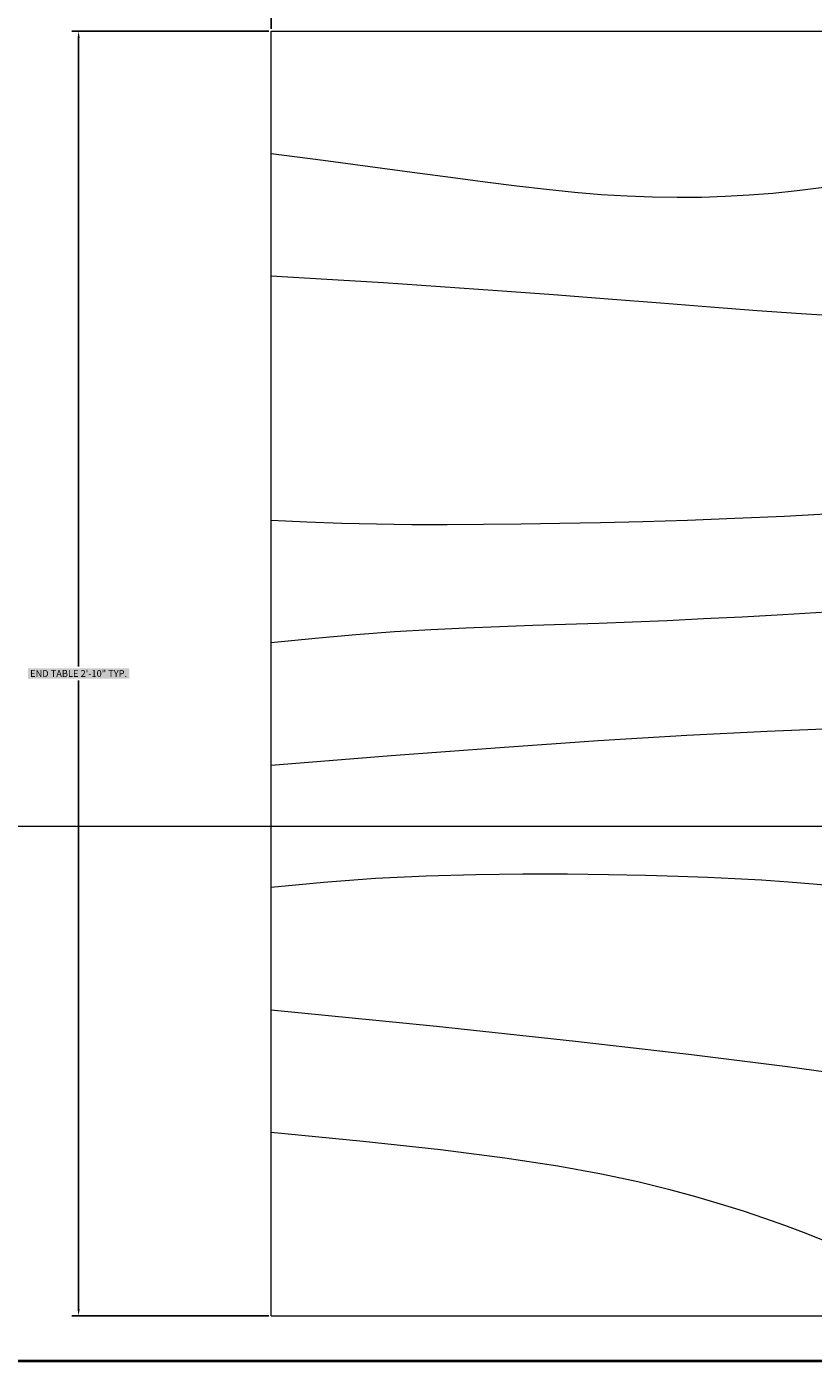
# Model space of a CAD drawing. Units: inches. Extents: x -301 to 715, y -607 to 364.
# Tile 100 of 141: x 82 to 103, y -10 to 26. Entities that reach past the tile are written whole.
import ezdxf

# ---------------------------------------------------------------- set-up
doc = ezdxf.new("R2010")
doc.units = ezdxf.units.IN
doc.header["$MEASUREMENT"] = 0
for name, color, linetype, lineweight in [('A-ANNO-DIMS', 2, 'Continuous', 18), ('A-FURN', 8, 'Continuous', 18), ('A-WALL', 3, 'Continuous', 40)]:
    doc.layers.add(name, color=color, linetype=linetype, lineweight=lineweight)
doc.styles.get("Standard").update_dxf_attribs({"font": 'arial.ttf'})
doc.dimstyles.get("Standard").update_dxf_attribs({"dimtxt": 0.18, "dimasz": 0.18, "dimexe": 0.18, "dimexo": 0.0625, "dimgap": 0.09, "dimtad": 0, "dimtih": 1, "dimtoh": 1, "dimdec": 1, "dimzin": 0, "dimdsep": 46, "dimlunit": 4, "dimtxsty": 'Standard', "dimcen": 0.09, "dimclrd": 3, "dimclre": 4, "dimclrt": 6, "dimadec": 0, "dimazin": 0, "dimtfac": 1, "dimtdec": 1, "dimtofl": 0, "dimtmove": 0, "dimatfit": 3, "dimfxl": 1, "dimtfill": 2, "dimtfillclr": 51, "dimtolj": 1, "dimtzin": 0, "dimarcsym": 0})

# ---------------------------------------------------------------- blocks, each defined once
blk = doc.blocks.new('Table - Square Woodgrain 42 x 42 in.')
blk.add_line((0, -42), (42, -42))
for points in [[(0, -4), (1.704, -4.2172), (3.2358, -4.4188), (4.615, -4.604), (5.8615, -4.7721), (6.9951, -4.9224), (8.0357, -5.0541), (9.0031, -5.1667), (9.9171, -5.2594), (10.7951, -5.3316), (11.6445, -5.3836), (12.4702, -5.4157), (13.277, -5.4283), (14.0698, -5.4217), (14.8535, -5.3964), (15.6331, -5.3526), (16.4133, -5.2908), (17.1986, -5.2103), (17.9913, -5.1062), (18.793, -4.9727), (19.6056, -4.8038), (20.4307, -4.5937), (21.2701, -4.3365), (22.1256, -4.0262), (22.9989, -3.6571), (23.888, -3.2272), (24.7756, -2.7516), (25.6408, -2.2491), (26.4624, -1.7387), (27.2195, -1.2395), (27.891, -0.7703), (28.456, -0.3501), (28.8934, 0.002)], [(0, -42), (0, 0), (42, 0), (42, -42)], [(0, -8), (1.8203, -8.1001), (3.6741, -8.2149), (5.5411, -8.3408), (7.4011, -8.4741), (9.2339, -8.6112), (11.0193, -8.7484), (12.7371, -8.8821), (14.3671, -9.0086), (15.8954, -9.1246), (17.3337, -9.2278), (18.6997, -9.3159), (20.0116, -9.387), (21.2871, -9.4389), (22.5442, -9.4696), (23.8008, -9.477), (25.0749, -9.459), (26.3791, -9.4137), (27.7049, -9.3403), (29.0383, -9.2382), (30.3655, -9.1068), (31.6728, -8.9455), (32.9461, -8.7535), (34.1717, -8.5304), (35.3358, -8.2756), (36.4268, -7.9863), (37.443, -7.6521), (38.3849, -7.2603), (39.253, -6.7986), (40.048, -6.2542), (40.7705, -5.6147), (41.421, -4.8674), (42, -4)], [(42, -12), (39.1784, -12.8621), (36.4519, -13.5654), (33.8246, -14.1294), (31.3004, -14.5731), (28.8832, -14.9161), (26.577, -15.1775), (24.3858, -15.3768), (22.3136, -15.5332), (20.3622, -15.6632), (18.5254, -15.7718), (16.7947, -15.8612), (15.1618, -15.9338), (13.6183, -15.9916), (12.1558, -16.0369), (10.7659, -16.0718), (9.4403, -16.0987), (8.1703, -16.1191), (6.9461, -16.1325), (5.7577, -16.1377), (4.595, -16.1335), (3.4479, -16.1188), (2.3064, -16.0924), (1.1604, -16.0532), (0, -16)], [(42, -16), (37.6529, -16.7365), (33.8802, -17.329), (30.6179, -17.7961), (27.8015, -18.1561), (25.3668, -18.4275), (23.2497, -18.6288), (21.3859, -18.7785), (19.7111, -18.8949), (18.1693, -18.9939), (16.7375, -19.0795), (15.401, -19.1534), (14.1449, -19.217), (12.9544, -19.2717), (11.8148, -19.3191), (10.7113, -19.3606), (9.6291, -19.3976), (8.5534, -19.4323), (7.47, -19.4689), (6.3643, -19.5122), (5.222, -19.5672), (4.0288, -19.6386), (2.7703, -19.7313), (1.4321, -19.8501), (0, -20)], [(0, -24), (3.9243, -23.6805), (7.4766, -23.4138), (10.6891, -23.1954), (13.5943, -23.0205), (16.2247, -22.8847), (18.6125, -22.7832), (20.7903, -22.7116), (22.7903, -22.6651), (24.6563, -22.642), (26.4764, -22.6507), (28.35, -22.7024), (30.3766, -22.8084), (32.6555, -22.98), (35.2861, -23.2283), (38.3678, -23.5645), (42, -24)], [(42, -32), (37.392, -31.017), (33.4585, -30.2231), (30.1291, -29.5949), (27.3334, -29.109), (25.0009, -28.742), (23.0612, -28.4707), (21.4439, -28.2716), (20.0786, -28.1215), (18.8998, -28.0002), (17.8609, -27.9014), (16.9206, -27.8219), (16.0371, -27.7588), (15.1691, -27.709), (14.2748, -27.6693), (13.3128, -27.6368), (12.2415, -27.6083), (11.0295, -27.5824), (9.6867, -27.5643), (8.233, -27.5608), (6.6884, -27.5787), (5.0728, -27.6248), (3.4062, -27.7058), (1.7086, -27.8286), (0, -28)], [(0, -32), (5.4026, -32.5358), (9.9494, -33.019), (13.7424, -33.4553), (16.8834, -33.8505), (19.4743, -34.2106), (21.6171, -34.5413), (23.4136, -34.8486), (24.9657, -35.1382), (26.3614, -35.4156), (27.6332, -35.6841), (28.7995, -35.9467), (29.8788, -36.2064), (30.8897, -36.4661), (31.8507, -36.7288), (32.7802, -36.9973), (33.6968, -37.2747), (34.6175, -37.5635), (35.5531, -37.8651), (36.5128, -38.1805), (37.506, -38.5108), (38.5421, -38.8568), (39.6302, -39.2197), (40.7797, -39.6004), (42, -40)], [(0, -36), (3.0098, -36.2857), (5.5354, -36.5643), (7.6368, -36.8359), (9.374, -37.1009), (10.807, -37.3597), (11.9957, -37.6126), (13.0002, -37.8599), (13.8804, -38.102), (14.6874, -38.3393), (15.4365, -38.5729), (16.1338, -38.8041), (16.7858, -39.0341), (17.3987, -39.264), (17.9787, -39.4952), (18.5322, -39.7288), (19.0655, -39.9662), (19.5832, -40.2081), (20.0842, -40.4544), (20.5657, -40.7046), (21.0249, -40.9581), (21.459, -41.2144), (21.8653, -41.4731), (22.2409, -41.7335), (22.5831, -41.9951)]]:
    blk.add_lwpolyline(points)
blk = doc.blocks.new('*D48')
at = {"layer": 'A-ANNO-DIMS', "color": 0, "lineweight": -2, "transparency": 16777216}
for p, q in [((-45.603, -7.657), (-45.603, 4.543)), ((122.71, -8.548), (122.71, 4.543))]:
    blk.add_line(p, q, dxfattribs=at)
at = {"layer": 'A-ANNO-DIMS', "color": 0, "lineweight": 0, "transparency": 16777216}
for p, q in [((-40.603, 4.363), (32.358, 4.363)), ((117.71, 4.363), (44.749, 4.363))]:
    blk.add_line(p, q, dxfattribs=at)
at = {"layer": 'A-ANNO-DIMS', "color": 0, "transparency": 16777216}
for points in [[(-40.603, 5.197), (-40.603, 3.53), (-45.603, 4.363)], [(117.71, 5.197), (117.71, 3.53), (122.71, 4.363)]]:
    blk.add_solid(points, dxfattribs=at)
at = {"layer": 'Defpoints', "color": 0, "transparency": 16777216}
for p in [(-45.603, 4.363), (-45.603, -7.72), (122.71, -8.61)]:
    blk.add_point(p, dxfattribs=at)
at = {"layer": 'A-ANNO-DIMS', "color": 0, "transparency": 16777216, "insert": (38.553, 4.363), "char_height": 3, "attachment_point": 5, "bg_fill": 1, "box_fill_scale": 1.25, "bg_fill_color": 51, "bg_fill_transparency": 0}
blk.add_mtext('\\A1;14\'-0{\\H1x;\\S1/2;}"', dxfattribs=at)
blk = doc.blocks.new('*D118')
at = {"layer": 'A-ANNO-DIMS', "color": 4, "lineweight": -2, "transparency": 16777216}
for p, q in [((88.597, 25.442), (83.372, 25.442)), ((88.597, -8.61), (83.372, -8.61))]:
    blk.add_line(p, q, dxfattribs=at)
at = {"layer": 'A-ANNO-DIMS', "color": 3, "lineweight": -2, "transparency": 16777216}
for p, q in [((83.552, 25.262), (83.552, 8.598)), ((83.552, -8.43), (83.552, 8.234))]:
    blk.add_line(p, q, dxfattribs=at)
at = {"layer": 'A-ANNO-DIMS', "color": 3, "transparency": 16777216}
for points in [[(83.522, 25.262), (83.582, 25.262), (83.552, 25.442)], [(83.522, -8.43), (83.582, -8.43), (83.552, -8.61)]]:
    blk.add_solid(points, dxfattribs=at)
at = {"layer": 'Defpoints', "color": 0, "transparency": 16777216}
for p in [(83.552, 25.442), (88.66, 25.442), (88.66, -8.61)]:
    blk.add_point(p, dxfattribs=at)
at = {"layer": 'A-ANNO-DIMS', "color": 6, "transparency": 16777216, "insert": (83.552, 8.416), "char_height": 0.18, "attachment_point": 5, "bg_fill": 1, "box_fill_scale": 1.25, "bg_fill_color": 51, "bg_fill_transparency": 0}
blk.add_mtext('\\A1;END TABLE 2\'-10" TYP.', dxfattribs=at)
blk = doc.blocks.new('*D119')
at = {"layer": 'A-ANNO-DIMS', "color": 4, "lineweight": -2, "transparency": 16777216}
for p, q in [((88.66, 25.504), (88.66, 30.729)), ((122.71, 25.504), (122.71, 30.729))]:
    blk.add_line(p, q, dxfattribs=at)
at = {"layer": 'A-ANNO-DIMS', "color": 3, "lineweight": -2, "transparency": 16777216}
for p, q in [((88.84, 30.549), (104.975, 30.549)), ((122.53, 30.549), (106.395, 30.549))]:
    blk.add_line(p, q, dxfattribs=at)
at = {"layer": 'A-ANNO-DIMS', "color": 3, "transparency": 16777216}
for points in [[(88.84, 30.579), (88.84, 30.519), (88.66, 30.549)], [(122.53, 30.579), (122.53, 30.519), (122.71, 30.549)]]:
    blk.add_solid(points, dxfattribs=at)
at = {"layer": 'Defpoints', "color": 0, "transparency": 16777216}
for p in [(122.71, 30.549), (88.66, 25.442), (122.71, 25.442)]:
    blk.add_point(p, dxfattribs=at)
at = {"layer": 'A-ANNO-DIMS', "color": 6, "transparency": 16777216, "insert": (105.685, 30.549), "char_height": 0.18, "attachment_point": 5, "bg_fill": 1, "box_fill_scale": 1.25, "bg_fill_color": 51, "bg_fill_transparency": 0}
blk.add_mtext('\\A1;2\'-10" TYP.', dxfattribs=at)

msp = doc.modelspace()

# ---------------------------------------------------------------- linework, layer by layer
at = {"layer": 'A-WALL'}
msp.add_line((123.897, -9.818), (21.897, -9.818), dxfattribs=at)

# ---------------------------------------------------------------- block references
at = {"layer": 'A-FURN', "xscale": 0.8107193059798699, "yscale": 0.8107193059798699, "zscale": 0.8107193059798699}
msp.add_blockref('Table - Square Woodgrain 42 x 42 in.', (88.66, 25.44), dxfattribs=at)

# ---------------------------------------------------------------- dimensions: what is measured, and where the dimension line sits
at = {"layer": 'A-ANNO-DIMS'}
dim = msp.add_linear_dim(base=(122.7099, 30.5493), p1=(88.6597, 25.4415), p2=(122.7099, 25.4415), text='<> TYP.', dimstyle='Standard', override={"dimdec": 1, "dimlfac": 1, "dimrnd": 0, "dimzin": 1, "dimdsep": 46, "dimlunit": 4, "dimfrac": 2}, dxfattribs=at)
dim.commit()
dim.dimension.update_dxf_attribs({"geometry": '*D119', "text_midpoint": (105.6848, 30.5493)})
dim = msp.add_linear_dim(base=(83.552, 25.442), p1=(88.66, -8.61), p2=(88.66, 25.442), angle=90, text='END TABLE <> TYP.', dimstyle='Standard', override={"dimdec": 1, "dimlfac": 1, "dimrnd": 0, "dimzin": 1, "dimdsep": 46, "dimlunit": 4, "dimfrac": 2}, dxfattribs=at)
dim.commit()
dim.dimension.update_dxf_attribs({"geometry": '*D118', "text_midpoint": (83.552, 8.416)})
dim = msp.add_linear_dim(base=(-45.603, 4.363), p1=(122.71, -8.61), p2=(-45.603, -7.72), dimstyle='Standard', override={"dimtxt": 3, "dimasz": 5, "dimclrd": 0, "dimclre": 0, "dimclrt": 0, "dimlwd": 0}, dxfattribs=at)
dim.commit()
dim.dimension.update_dxf_attribs({"geometry": '*D48', "text_midpoint": (38.553, 4.363)})

doc.saveas('drawing.dxf')
